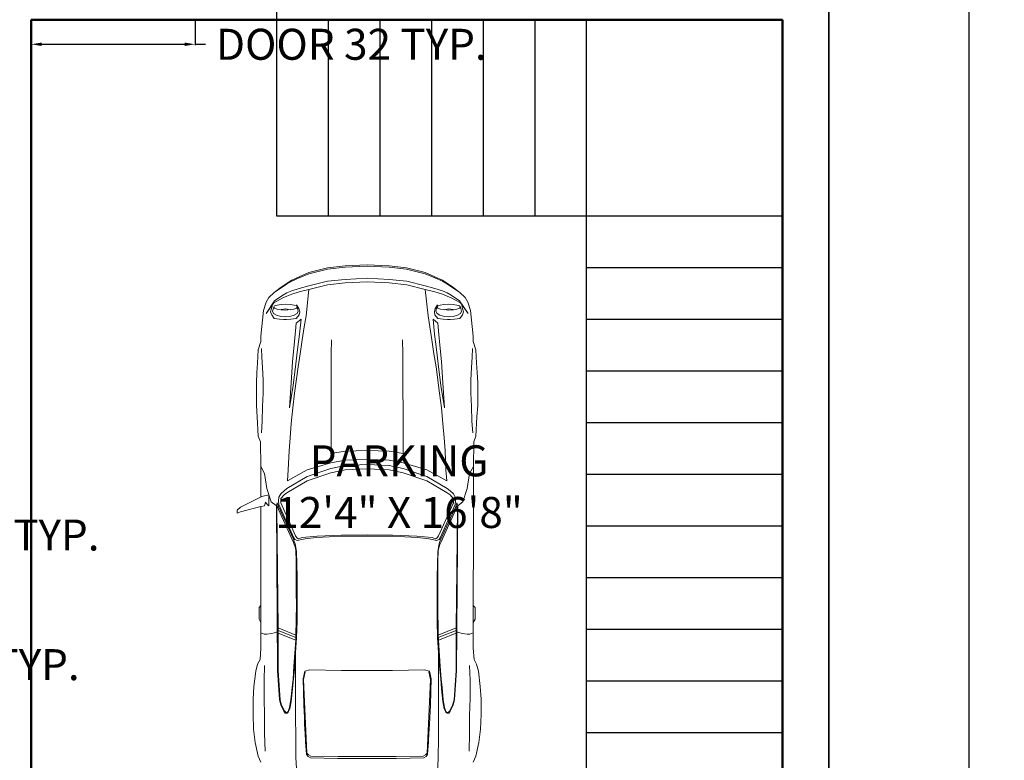
# Model space of a CAD drawing. Units: inches. Extents: x -20 to 10156, y 488 to 2970.
# Tile 3 of 6: x 221 to 412, y 581 to 724. Entities that reach past the tile are written whole.
import ezdxf

# ---------------------------------------------------------------- set-up
doc = ezdxf.new("R2010")
doc.units = ezdxf.units.IN
doc.header["$MEASUREMENT"] = 0
for name, color, linetype, lineweight in [('A-ANNO-DIMS', 2, 'Continuous', 18), ('A-AREA-IDEN', 7, 'Continuous', 25), ('A-FLOR-STRS', 7, 'Continuous', 25), ('A-FURN-VEHC', 8, 'Continuous', 13), ('A-WALL', 7, 'Continuous', 50), ('C-PROP', 7, 'Continuous', 35)]:
    doc.layers.add(name, color=color, linetype=linetype, lineweight=lineweight)
doc.styles.get("Standard").update_dxf_attribs({"font": 'arial.ttf'})
doc.dimstyles.get("Standard").update_dxf_attribs({"dimtxt": 6, "dimasz": 2, "dimexe": 0.18, "dimexo": 0.0625, "dimgap": 0.09, "dimtad": 0, "dimtih": 1, "dimtoh": 1, "dimdec": 0, "dimzin": 0, "dimdsep": 46, "dimlunit": 4, "dimtxsty": 'Standard', "dimcen": 0.09, "dimadec": 0, "dimazin": 0, "dimtfac": 1, "dimtdec": 0, "dimtofl": 0, "dimtmove": 0, "dimatfit": 3, "dimfxl": 1, "dimtolj": 1, "dimtzin": 0, "dimarcsym": 0})

# ---------------------------------------------------------------- blocks, each defined once
blk = doc.blocks.new('*D12')
at = {"layer": 'A-ANNO-DIMS', "color": 0, "lineweight": -2, "transparency": 16777216}
for p, q in [((223.3, 724.17), (223.3, 719.29)), ((255.01, 724.17), (255.01, 719.29)), ((225.3, 719.47), (253.01, 719.47)), ((255.01, 719.47), (257.01, 719.47))]:
    blk.add_line(p, q, dxfattribs=at)
at = {"layer": 'A-ANNO-DIMS', "color": 0, "transparency": 16777216}
for points in [[(225.3, 719.81), (225.3, 719.14), (223.3, 719.47)], [(253.01, 719.81), (253.01, 719.14), (255.01, 719.47)]]:
    blk.add_solid(points, dxfattribs=at)
at = {"layer": 'Defpoints', "color": 0, "transparency": 16777216}
for p in [(223.3, 724.23), (255.01, 724.23), (255.01, 719.47)]:
    blk.add_point(p, dxfattribs=at)
at = {"layer": 'A-ANNO-DIMS', "color": 0, "transparency": 16777216, "insert": (285.29, 719.47), "char_height": 6, "attachment_point": 5}
blk.add_mtext('\\A1;DOOR 32 TYP.', dxfattribs=at)
blk = doc.blocks.new('*D14')
at = {"layer": 'A-ANNO-DIMS', "color": 0, "lineweight": -2, "transparency": 16777216}
for p, q in [((206, 618.67), (211.91, 618.67)), ((211.73, 616.67), (211.73, 602.56)), ((211.73, 582.06), (211.73, 596.17)), ((206, 580.06), (211.91, 580.06))]:
    blk.add_line(p, q, dxfattribs=at)
at = {"layer": 'A-ANNO-DIMS', "color": 0, "transparency": 16777216}
for points in [[(211.4, 616.67), (212.07, 616.67), (211.73, 618.67)], [(211.4, 582.06), (212.07, 582.06), (211.73, 580.06)]]:
    blk.add_solid(points, dxfattribs=at)
at = {"layer": 'Defpoints', "color": 0, "transparency": 16777216}
for p in [(205.94, 618.67), (205.94, 580.06), (211.73, 580.06)]:
    blk.add_point(p, dxfattribs=at)
at = {"layer": 'A-ANNO-DIMS', "color": 0, "transparency": 16777216, "insert": (211.73, 599.36), "char_height": 6, "attachment_point": 5}
blk.add_mtext('\\A1;WC 39 TYP.', dxfattribs=at)
blk = doc.blocks.new('*D15')
at = {"layer": 'A-ANNO-DIMS', "color": 0, "lineweight": -2, "transparency": 16777216}
for p, q in [((181.78, 618.73), (181.78, 624.64)), ((183.78, 624.46), (203.94, 624.46)), ((205.94, 618.73), (205.94, 624.64)), ((205.94, 624.46), (207.94, 624.46))]:
    blk.add_line(p, q, dxfattribs=at)
at = {"layer": 'A-ANNO-DIMS', "color": 0, "transparency": 16777216}
for points in [[(183.78, 624.79), (183.78, 624.13), (181.78, 624.46)], [(203.94, 624.79), (203.94, 624.13), (205.94, 624.46)]]:
    blk.add_solid(points, dxfattribs=at)
at = {"layer": 'Defpoints', "color": 0, "transparency": 16777216}
for p in [(205.94, 624.46), (181.78, 618.67), (205.94, 618.67)]:
    blk.add_point(p, dxfattribs=at)
at = {"layer": 'A-ANNO-DIMS', "color": 0, "transparency": 16777216, "insert": (222.69, 624.46), "char_height": 6, "attachment_point": 5}
blk.add_mtext('\\A1;24 TYP.', dxfattribs=at)
blk = doc.blocks.new('*D29')
at = {"layer": 'A-ANNO-DIMS', "color": 0, "lineweight": -2, "transparency": 16777216}
for p, q in [((377.86, 1058.73), (405.13, 1058.73)), ((404.95, 1056.73), (404.95, 791.88)), ((404.95, 520.73), (404.95, 785.58)), ((377.86, 518.73), (405.13, 518.73))]:
    blk.add_line(p, q, dxfattribs=at)
at = {"layer": 'A-ANNO-DIMS', "color": 0, "transparency": 16777216}
for points in [[(404.62, 1056.73), (405.28, 1056.73), (404.95, 1058.73)], [(404.62, 520.73), (405.28, 520.73), (404.95, 518.73)]]:
    blk.add_solid(points, dxfattribs=at)
at = {"layer": 'Defpoints', "color": 0, "transparency": 16777216}
for p in [(377.8, 1058.73), (404.95, 1058.73), (377.8, 518.73)]:
    blk.add_point(p, dxfattribs=at)
at = {"layer": 'A-ANNO-DIMS', "color": 0, "transparency": 16777216, "insert": (404.95, 788.73), "char_height": 6, "attachment_point": 5}
blk.add_mtext('\\A1;540', dxfattribs=at)

msp = doc.modelspace()

# ---------------------------------------------------------------- linework, layer by layer
at = {"layer": 'A-FLOR-STRS'}
for p, q in [((270.8, 728.73), (270.8, 686.23)), ((280.8, 724.23), (280.8, 686.23)), ((290.8, 724.23), (290.8, 686.23)), ((300.8, 724.23), (300.8, 686.23)), ((310.8, 724.23), (310.8, 686.23)), ((320.8, 724.23), (320.8, 686.23)), ((330.8, 724.23), (330.8, 676.23)), ((270.8, 686.23), (368.8, 686.23)), ((330.8, 676.23), (368.8, 676.23)), ((330.8, 676.23), (330.8, 566.23)), ((330.8, 666.23), (368.8, 666.23)), ((330.8, 656.23), (368.8, 656.23)), ((330.8, 646.23), (368.8, 646.23)), ((330.8, 636.23), (368.8, 636.23)), ((330.8, 626.23), (368.8, 626.23)), ((330.8, 616.23), (368.8, 616.23)), ((330.8, 606.23), (368.8, 606.23)), ((330.8, 596.23), (368.8, 596.23)), ((330.8, 586.23), (368.8, 586.23))]:
    msp.add_line(p, q, dxfattribs=at)
at = {"layer": 'A-FURN-VEHC'}
for p, q in [((277.07, 675.28, -279.43), (275.2, 674.47, -279.43)), ((280.66, 676.17, -279.43), (277.07, 675.28, -279.43)), ((280.66, 675.92, -279.43), (277.07, 675.02, -279.43)), ((284.07, 676.56, -279.43), (280.66, 676.17, -279.43)), ((284.07, 676.3, -279.43), (280.66, 675.92, -279.43)), ((288.33, 676.77, -279.43), (284.07, 676.56, -279.43)), ((288.33, 676.52, -279.43), (284.07, 676.3, -279.43)), ((288.33, 676.77, -279.43), (288.33, 676.77, -279.43)), ((288.33, 676.77, -279.43), (292.59, 676.56, -279.43)), ((288.33, 676.52, -279.43), (292.59, 676.3, -279.43)), ((292.59, 676.56, -279.43), (296, 676.17, -279.43)), ((292.59, 676.3, -279.43), (296, 675.92, -279.43)), ((296, 676.17, -279.43), (299.59, 675.28, -279.43)), ((296, 675.92, -279.43), (299.59, 675.02, -279.43)), ((299.59, 675.28, -279.43), (301.46, 674.47, -279.43)), ((273.75, 673.83, -279.43), (271.71, 672.43, -279.43)), ((273.75, 673.58, -279.43), (272.72, 673.02, -279.43)), ((275.2, 674.47, -279.43), (273.75, 673.83, -279.43)), ((275.2, 674.22, -279.43), (273.75, 673.58, -279.43)), ((277.07, 675.02, -279.43), (275.2, 674.22, -279.43)), ((277.06, 672.68, -279.43), (280.65, 673.58, -279.43)), ((280.65, 673.58, -279.43), (284.06, 673.96, -279.43)), ((284.06, 673.27, -279.43), (280.65, 672.89, -279.43)), ((284.06, 673.96, -279.43), (288.33, 674.17, -279.43)), ((288.33, 673.48, -279.43), (284.06, 673.27, -279.43)), ((292.6, 673.96, -279.43), (288.33, 674.17, -279.43)), ((288.33, 673.48, -279.43), (292.6, 673.27, -279.43)), ((296.01, 673.58, -279.43), (292.6, 673.96, -279.43)), ((292.6, 673.27, -279.43), (296.01, 672.89, -279.43)), ((299.6, 672.68, -279.43), (296.01, 673.58, -279.43)), ((299.59, 675.02, -279.43), (301.46, 674.22, -279.43)), ((301.46, 674.47, -279.43), (302.92, 673.83, -279.43)), ((301.46, 674.22, -279.43), (302.92, 673.58, -279.43)), ((302.92, 673.83, -279.43), (304.95, 672.43, -279.43)), ((302.92, 673.58, -279.43), (303.94, 673.02, -279.43)), ((270.33, 671.4, -279.43), (269.31, 670.46, -279.43)), ((272.72, 673.02, -279.43), (270.33, 671.4, -279.43)), ((271.71, 672.43, -279.43), (270.33, 671.4, -279.43)), ((272.03, 670.89, -279.43), (272.79, 671.32, -279.43)), ((272.79, 671.32, -279.43), (273.73, 671.74, -279.43)), ((273.73, 671.74, -279.43), (275.19, 672.2, -279.43)), ((275.19, 671.53, -279.43), (273.73, 671.06, -279.43)), ((275.19, 672.2, -279.43), (277.06, 672.68, -279.43)), ((277.06, 671.99, -279.43), (275.19, 671.53, -279.43)), ((277.06, 671.99, -279.43), (276.53, 666.9, -279.43)), ((280.65, 672.89, -279.43), (277.06, 671.99, -279.43)), ((296.01, 672.89, -279.43), (299.6, 671.99, -279.43)), ((301.47, 672.2, -279.43), (299.6, 672.68, -279.43)), ((299.6, 671.99, -279.43), (301.47, 671.53, -279.43)), ((299.6, 671.99, -279.43), (300.14, 666.9, -279.43)), ((302.93, 671.74, -279.43), (301.47, 672.2, -279.43)), ((301.47, 671.53, -279.43), (302.93, 671.06, -279.43)), ((303.87, 671.32, -279.43), (302.93, 671.74, -279.43)), ((304.63, 670.89, -279.43), (303.87, 671.32, -279.43)), ((303.94, 673.02, -279.43), (306.33, 671.4, -279.43)), ((304.95, 672.43, -279.43), (306.33, 671.4, -279.43)), ((306.33, 671.4, -279.43), (307.35, 670.46, -279.43)), ((268.8, 669.53, -279.43), (268.29, 667.9, -279.43)), ((268.76, 667.37, -279.43), (270.4, 669.78, -279.43)), ((270.25, 669.43, -279.43), (268.76, 667.37, -279.43)), ((269.31, 670.46, -279.43), (268.8, 669.53, -279.43)), ((272.03, 670.38, -279.43), (270.25, 669.43, -279.43)), ((270.4, 669.78, -279.43), (272.03, 670.89, -279.43)), ((272.79, 670.71, -279.43), (272.03, 670.38, -279.43)), ((273.73, 671.06, -279.43), (272.79, 670.71, -279.43)), ((302.93, 671.06, -279.43), (303.87, 670.71, -279.43)), ((303.87, 670.71, -279.43), (304.63, 670.38, -279.43)), ((306.26, 669.78, -279.43), (304.63, 670.89, -279.43)), ((304.63, 670.38, -279.43), (306.41, 669.43, -279.43)), ((307.9, 667.37, -279.43), (306.26, 669.78, -279.43)), ((306.41, 669.43, -279.43), (307.9, 667.37, -279.43)), ((307.35, 670.46, -279.43), (307.86, 669.53, -279.43)), ((307.86, 669.53, -279.43), (308.38, 667.9, -279.43)), ((268.29, 667.9, -279.43), (267.77, 662.95, -279.43)), ((269.82, 668.33, -279.43), (269.66, 667.64, -279.43)), ((269.66, 667.64, -279.43), (269.87, 667.07, -279.43)), ((270, 669.01, -279.43), (269.82, 668.33, -279.43)), ((270.01, 667.78, -279.43), (270.25, 668.58, -279.43)), ((270.21, 667.35, -279.43), (270.01, 667.78, -279.43)), ((270.43, 668.8, -279.43), (270.25, 668.58, -279.43)), ((270.25, 668.58, -279.43), (270.43, 668.39, -279.43)), ((270.93, 668.98, -279.43), (270.43, 668.8, -279.43)), ((270.43, 668.39, -279.43), (270.93, 668.2, -279.43)), ((271.67, 669.11, -279.43), (270.93, 668.98, -279.43)), ((270.93, 668.2, -279.43), (271.6, 668.08, -279.43)), ((271.6, 668.08, -279.43), (272.56, 668.02, -279.43)), ((272.56, 669.14, -279.43), (271.67, 669.11, -279.43)), ((271.67, 668.11, -279.43), (272.56, 668.22, -279.43)), ((273.43, 669.11, -279.43), (272.56, 669.14, -279.43)), ((272.56, 668.22, -279.43), (273.42, 668.07, -279.43)), ((272.56, 668.02, -279.43), (273.43, 668.11, -279.43)), ((274.19, 668.98, -279.43), (273.43, 669.11, -279.43)), ((273.43, 668.11, -279.43), (274.13, 668.19, -279.43)), ((274.13, 668.19, -279.43), (274.64, 668.37, -279.43)), ((274.65, 668.8, -279.43), (274.19, 668.98, -279.43)), ((274.64, 668.37, -279.43), (274.8, 668.58, -279.43)), ((274.8, 668.58, -279.43), (274.65, 668.8, -279.43)), ((275.12, 668.33, -279.43), (274.69, 669.01, -279.43)), ((274.99, 667.78, -279.43), (274.77, 667.35, -279.43)), ((274.8, 668.58, -279.43), (274.94, 668.04, -279.43)), ((274.94, 668.04, -279.43), (274.99, 667.78, -279.43)), ((275.28, 667.64, -279.43), (275.12, 668.33, -279.43)), ((275.21, 667.07, -279.43), (275.28, 667.64, -279.43)), ((301.38, 667.64, -279.43), (301.54, 668.33, -279.43)), ((301.45, 667.07, -279.43), (301.38, 667.64, -279.43)), ((301.54, 668.33, -279.43), (301.97, 669.01, -279.43)), ((301.72, 668.04, -279.43), (301.67, 667.78, -279.43)), ((301.67, 667.78, -279.43), (301.89, 667.35, -279.43)), ((301.86, 668.58, -279.43), (301.72, 668.04, -279.43)), ((301.86, 668.58, -279.43), (302.01, 668.8, -279.43)), ((302.02, 668.37, -279.43), (301.86, 668.58, -279.43)), ((302.01, 668.8, -279.43), (302.48, 668.98, -279.43)), ((302.53, 668.19, -279.43), (302.02, 668.37, -279.43)), ((302.48, 668.98, -279.43), (303.23, 669.11, -279.43)), ((303.23, 668.11, -279.43), (302.53, 668.19, -279.43)), ((303.23, 669.11, -279.43), (304.1, 669.14, -279.43)), ((304.1, 668.02, -279.43), (303.23, 668.11, -279.43)), ((304.1, 668.22, -279.43), (303.24, 668.07, -279.43)), ((304.1, 669.14, -279.43), (304.99, 669.11, -279.43)), ((304.99, 668.11, -279.43), (304.1, 668.22, -279.43)), ((305.06, 668.08, -279.43), (304.1, 668.02, -279.43)), ((304.99, 669.11, -279.43), (305.73, 668.98, -279.43)), ((305.73, 668.2, -279.43), (305.06, 668.08, -279.43)), ((305.73, 668.98, -279.43), (306.24, 668.8, -279.43)), ((306.24, 668.39, -279.43), (305.73, 668.2, -279.43)), ((306.24, 668.8, -279.43), (306.41, 668.58, -279.43)), ((306.41, 668.58, -279.43), (306.24, 668.39, -279.43)), ((306.65, 667.78, -279.43), (306.41, 668.58, -279.43)), ((306.46, 667.35, -279.43), (306.65, 667.78, -279.43)), ((306.67, 669.01, -279.43), (306.84, 668.33, -279.43)), ((307, 667.64, -279.43), (306.79, 667.07, -279.43)), ((306.84, 668.33, -279.43), (307, 667.64, -279.43)), ((308.38, 667.9, -279.43), (308.89, 662.95, -279.43)), ((269.87, 667.07, -279.43), (270.33, 666.39, -279.43)), ((270.8, 667.01, -279.43), (270.21, 667.35, -279.43)), ((270.33, 666.39, -279.43), (271.36, 666.22, -279.43)), ((271.66, 666.78, -279.43), (270.8, 667.01, -279.43)), ((271.36, 666.22, -279.43), (272.21, 666.19, -279.43)), ((272.51, 666.7, -279.43), (271.66, 666.78, -279.43)), ((272.21, 666.19, -279.43), (272.72, 666.19, -279.43)), ((273.36, 666.78, -279.43), (272.51, 666.7, -279.43)), ((272.72, 666.19, -279.43), (273.58, 666.22, -279.43)), ((274.22, 667.01, -279.43), (273.36, 666.78, -279.43)), ((273.58, 666.22, -279.43), (274.61, 666.39, -279.43)), ((274.77, 667.35, -279.43), (274.22, 667.01, -279.43)), ((274.61, 666.39, -279.43), (275.21, 667.07, -279.43)), ((275.55, 666.24, -279.43), (274.62, 665.48, -279.43)), ((275.25, 663.32, -279.43), (275.55, 666.24, -279.43)), ((276.53, 666.9, -279.43), (276.18, 664.79, -279.43)), ((300.14, 666.9, -279.43), (300.48, 664.79, -279.43)), ((301.42, 663.32, -279.43), (301.11, 666.24, -279.43)), ((301.11, 666.24, -279.43), (302.04, 665.48, -279.43)), ((302.06, 666.39, -279.43), (301.45, 667.07, -279.43)), ((301.89, 667.35, -279.43), (302.44, 667.01, -279.43)), ((303.08, 666.22, -279.43), (302.06, 666.39, -279.43)), ((302.44, 667.01, -279.43), (303.3, 666.78, -279.43)), ((303.94, 666.19, -279.43), (303.08, 666.22, -279.43)), ((303.3, 666.78, -279.43), (304.15, 666.7, -279.43)), ((304.45, 666.19, -279.43), (303.94, 666.19, -279.43)), ((304.15, 666.7, -279.43), (305, 666.78, -279.43)), ((305.3, 666.22, -279.43), (304.45, 666.19, -279.43)), ((305, 666.78, -279.43), (305.86, 667.01, -279.43)), ((306.33, 666.39, -279.43), (305.3, 666.22, -279.43)), ((305.86, 667.01, -279.43), (306.46, 667.35, -279.43)), ((306.79, 667.07, -279.43), (306.33, 666.39, -279.43)), ((274.49, 663.96, -279.43), (274.22, 661.19, -279.43)), ((274.62, 665.48, -279.43), (274.49, 663.96, -279.43)), ((276.18, 664.79, -279.43), (275.78, 662.26, -279.43)), ((300.48, 664.79, -279.43), (300.88, 662.26, -279.43)), ((302.04, 665.48, -279.43), (302.17, 663.96, -279.43)), ((302.17, 663.96, -279.43), (302.44, 661.19, -279.43)), ((267.77, 661.92, -279.43), (267.27, 660.31, -279.43)), ((267.77, 662.95, -279.43), (267.77, 661.92, -279.43)), ((274.87, 660.4, -279.43), (275.25, 663.32, -279.43)), ((275.78, 662.26, -279.43), (275.37, 659.52, -279.43)), ((281.4, 659.52, -279.43), (281.44, 662.26, -279.43)), ((295.26, 659.52, -279.43), (295.22, 662.26, -279.43)), ((300.88, 662.26, -279.43), (301.29, 659.52, -279.43)), ((301.79, 660.4, -279.43), (301.42, 663.32, -279.43)), ((308.89, 662.95, -279.43), (308.89, 661.92, -279.43)), ((308.89, 661.92, -279.43), (309.39, 660.31, -279.43)), ((267.27, 660.31, -279.43), (267.12, 657.75, -279.43)), ((267.89, 660.56, -279.43), (267.97, 658.86, -279.43)), ((274.22, 661.19, -279.43), (273.92, 658.03, -279.43)), ((274.54, 657.57, -279.43), (274.87, 660.4, -279.43)), ((302.13, 657.57, -279.43), (301.79, 660.4, -279.43)), ((302.44, 661.19, -279.43), (302.74, 658.03, -279.43)), ((308.77, 660.56, -279.43), (308.69, 658.86, -279.43)), ((309.39, 660.31, -279.43), (309.54, 657.75, -279.43)), ((267.97, 658.86, -279.43), (268.09, 656.9, -279.43)), ((273.92, 658.03, -279.43), (273.7, 654.86, -279.43)), ((275.37, 659.52, -279.43), (274.97, 657.05, -279.43)), ((281.35, 641.81, -279.43), (281.4, 659.52, -279.43)), ((295.32, 641.81, -279.43), (295.26, 659.52, -279.43)), ((301.29, 659.52, -279.43), (301.7, 657.05, -279.43)), ((302.74, 658.03, -279.43), (302.96, 654.86, -279.43)), ((308.69, 658.86, -279.43), (308.57, 656.9, -279.43)), ((267.12, 657.75, -279.43), (266.98, 655.95, -279.43)), ((268.09, 656.9, -279.43), (268.2, 654.43, -279.43)), ((274.05, 653.4, -279.43), (274.54, 657.57, -279.43)), ((274.97, 657.05, -279.43), (274.28, 651.95, -279.43)), ((301.7, 657.05, -279.43), (302.38, 651.95, -279.43)), ((302.61, 653.4, -279.43), (302.13, 657.57, -279.43)), ((308.57, 656.9, -279.43), (308.46, 654.43, -279.43)), ((309.54, 657.75, -279.43), (309.68, 655.95, -279.43)), ((266.98, 655.95, -279.43), (266.9, 653.92, -279.43)), ((268.2, 654.43, -279.43), (268.23, 651.95, -279.43)), ((273.7, 654.86, -279.43), (273.31, 649.05, -279.43)), ((302.96, 654.86, -279.43), (303.35, 649.05, -279.43)), ((308.46, 654.43, -279.43), (308.44, 651.95, -279.43)), ((309.68, 655.95, -279.43), (309.76, 653.92, -279.43)), ((266.9, 653.92, -279.43), (266.9, 651.95, -279.43)), ((273.31, 649.05, -279.43), (274.05, 653.4, -279.43)), ((303.35, 649.05, -279.43), (302.61, 653.4, -279.43)), ((309.76, 653.92, -279.43), (309.76, 651.95, -279.43)), ((266.9, 651.95, -279.43), (266.9, 649.56, -279.43)), ((268.23, 651.95, -279.43), (268.11, 649.34, -279.43)), ((274.28, 651.95, -279.43), (273.94, 649.05, -279.43)), ((302.38, 651.95, -279.43), (302.72, 649.05, -279.43)), ((308.44, 651.95, -279.43), (308.55, 649.34, -279.43)), ((309.76, 651.95, -279.43), (309.76, 649.56, -279.43)), ((266.9, 649.56, -279.43), (267.04, 647.34, -279.43)), ((268.11, 649.34, -279.43), (268.03, 646.49, -279.43)), ((273.94, 649.05, -279.43), (273.66, 646.06, -279.43)), ((302.72, 649.05, -279.43), (303, 646.06, -279.43)), ((308.55, 649.34, -279.43), (308.63, 646.49, -279.43)), ((309.76, 649.56, -279.43), (309.62, 647.34, -279.43)), ((267.04, 647.34, -279.43), (267.27, 643.59, -279.43)), ((309.62, 647.34, -279.43), (309.39, 643.59, -279.43)), ((268.03, 646.49, -279.43), (267.87, 644.24, -279.43)), ((273.66, 646.06, -279.43), (273.41, 643.25, -279.43)), ((303, 646.06, -279.43), (303.25, 643.25, -279.43)), ((308.63, 646.49, -279.43), (308.8, 644.24, -279.43)), ((267.27, 643.59, -279.43), (267.67, 642.47, -279.43)), ((273.41, 643.25, -279.43), (273.23, 640.77, -279.43)), ((303.25, 643.25, -279.43), (303.43, 640.77, -279.43)), ((309.39, 643.59, -279.43), (308.99, 642.47, -279.43)), ((267.67, 642.47, -279.43), (267.74, 637.7, -279.43)), ((281.33, 640.25, -279.43), (281.35, 641.81, -279.43)), ((288.33, 640.84, -279.43), (284.07, 640.67, -279.43)), ((288.33, 640.84, -279.43), (292.59, 640.67, -279.43)), ((295.33, 640.25, -279.43), (295.32, 641.81, -279.43)), ((308.99, 642.47, -279.43), (308.92, 637.7, -279.43)), ((273.23, 640.77, -279.43), (273.07, 637.08, -279.43)), ((284.07, 640.67, -279.43), (281.33, 640.25, -279.43)), ((281.33, 638.41, -279.43), (284.07, 638.92, -279.43)), ((284.07, 638.92, -279.43), (288.33, 639.1, -279.43)), ((292.59, 638.92, -279.43), (288.33, 639.1, -279.43)), ((292.59, 640.67, -279.43), (295.33, 640.25, -279.43)), ((295.33, 638.41, -279.43), (292.59, 638.92, -279.43)), ((303.43, 640.77, -279.43), (303.59, 637.08, -279.43)), ((267.74, 637.7, -279.43), (267.73, 631.8, -279.43)), ((268.46, 636.34, -279.43), (267.74, 637.7, -279.43)), ((273.07, 637.08, -279.43), (272.9, 634.93, -279.43)), ((272.9, 634.93, -279.43), (276.73, 637.05, -279.43)), ((276.73, 637.05, -279.43), (281.33, 638.41, -279.43)), ((281.33, 637.34, -279.43), (276.73, 635.8, -279.43)), ((284.07, 637.93, -279.43), (281.33, 637.34, -279.43)), ((284.07, 637.07, -279.43), (281.33, 636.48, -279.43)), ((288.33, 638.11, -279.43), (284.07, 637.93, -279.43)), ((288.33, 637.25, -279.43), (284.07, 637.07, -279.43)), ((288.33, 638.11, -279.43), (292.59, 637.93, -279.43)), ((288.33, 637.25, -279.43), (292.59, 637.07, -279.43)), ((292.59, 637.93, -279.43), (295.33, 637.34, -279.43)), ((292.59, 637.07, -279.43), (295.33, 636.48, -279.43)), ((299.94, 637.05, -279.43), (295.33, 638.41, -279.43)), ((295.33, 637.34, -279.43), (299.94, 635.8, -279.43)), ((303.77, 634.93, -279.43), (299.94, 637.05, -279.43)), ((303.59, 637.08, -279.43), (303.77, 634.93, -279.43)), ((308.2, 636.34, -279.43), (308.92, 637.7, -279.43)), ((308.92, 637.7, -279.43), (308.94, 631.8, -279.43)), ((268.91, 633.44, -279.43), (268.46, 636.34, -279.43)), ((276.73, 635.8, -279.43), (272.81, 633.44, -279.43)), ((281.33, 636.48, -279.43), (276.73, 634.94, -279.43)), ((295.33, 636.48, -279.43), (299.94, 634.94, -279.43)), ((299.94, 635.8, -279.43), (303.85, 633.44, -279.43)), ((307.75, 633.44, -279.43), (308.2, 636.34, -279.43)), ((269.78, 630.88, -279.43), (268.91, 633.44, -279.43)), ((272.81, 633.44, -279.43), (272.25, 633.03, -279.43)), ((276.73, 634.94, -279.43), (272.81, 632.61, -279.43)), ((299.94, 634.94, -279.43), (303.85, 632.61, -279.43)), ((303.85, 633.44, -279.43), (304.41, 633.03, -279.43)), ((306.89, 630.88, -279.43), (307.75, 633.44, -279.43)), ((267.95, 631.9, -279.43), (263.85, 629.85, -279.43)), ((269.31, 632.24, -279.43), (267.95, 631.9, -279.43)), ((269.31, 630.11, -279.43), (269.31, 632.24, -279.43)), ((271.27, 631.77, -279.43), (271.21, 631.1, -279.43)), ((271.61, 632.41, -279.43), (271.27, 631.77, -279.43)), ((271.66, 631.55, -279.43), (271.6, 630.68, -279.43)), ((272.25, 633.03, -279.43), (271.61, 632.41, -279.43)), ((272.25, 632.24, -279.43), (271.66, 631.55, -279.43)), ((272.81, 632.61, -279.43), (272.25, 632.24, -279.43)), ((303.85, 632.61, -279.43), (304.41, 632.24, -279.43)), ((304.41, 633.03, -279.43), (305.05, 632.41, -279.43)), ((304.41, 632.24, -279.43), (305, 631.55, -279.43)), ((305, 631.55, -279.43), (305.06, 630.68, -279.43)), ((305.05, 632.41, -279.43), (305.4, 631.77, -279.43)), ((305.4, 631.77, -279.43), (305.46, 631.1, -279.43)), ((308.92, 629.96, -279.43), (308.94, 631.8, -279.43)), ((263.85, 629.85, -279.43), (263.18, 629.26, -279.43)), ((263.85, 628.92, -279.43), (267.75, 629.96, -279.43)), ((267.74, 629.96, -279.43), (267.78, 605.55, -279.43)), ((267.75, 629.96, -279.43), (268.46, 630.13, -279.43)), ((268.46, 630.13, -279.43), (268.63, 630.8, -279.43)), ((268.63, 630.8, -279.43), (269.04, 630.3, -279.43)), ((269.04, 630.3, -279.43), (269.31, 630.11, -279.43)), ((270.7, 630.19, -279.43), (269.78, 630.88, -279.43)), ((270.76, 630.19, -279.43), (270.94, 630.67, -279.43)), ((271.01, 598.2, -279.43), (270.76, 630.19, -279.43)), ((270.85, 629.82, -279.43), (270.94, 630.08, -279.43)), ((270.97, 617.72, -279.43), (270.85, 629.82, -279.43)), ((270.94, 630.67, -279.43), (271.16, 630.01, -279.43)), ((270.94, 630.08, -279.43), (271.16, 629.4, -279.43)), ((271.16, 630.01, -279.43), (274.06, 623.65, -279.43)), ((271.16, 629.4, -279.43), (274.06, 623.04, -279.43)), ((271.21, 631.1, -279.43), (271.23, 630.37, -279.43)), ((271.23, 630.37, -279.43), (274.15, 623.94, -279.43)), ((271.6, 630.68, -279.43), (274.5, 624.29, -279.43)), ((305.06, 630.68, -279.43), (302.16, 624.29, -279.43)), ((305.43, 630.37, -279.43), (302.51, 623.94, -279.43)), ((305.5, 630.01, -279.43), (302.6, 623.65, -279.43)), ((305.5, 629.4, -279.43), (302.6, 623.04, -279.43)), ((305.46, 631.1, -279.43), (305.43, 630.37, -279.43)), ((305.72, 630.67, -279.43), (305.5, 630.01, -279.43)), ((305.72, 630.08, -279.43), (305.5, 629.4, -279.43)), ((305.65, 598.2, -279.43), (305.9, 630.19, -279.43)), ((305.69, 617.72, -279.43), (305.82, 629.82, -279.43)), ((305.9, 630.19, -279.43), (305.72, 630.67, -279.43)), ((305.82, 629.82, -279.43), (305.72, 630.08, -279.43)), ((305.97, 630.19, -279.43), (306.89, 630.88, -279.43)), ((308.92, 629.96, -279.43), (308.88, 605.55, -279.43)), ((263.18, 629.26, -279.43), (263.18, 628.67, -279.43)), ((263.18, 628.67, -279.43), (263.85, 628.92, -279.43)), ((274.06, 623.65, -279.43), (274.22, 623.22, -279.43)), ((274.15, 623.94, -279.43), (274.35, 623.56, -279.43)), ((274.5, 624.29, -279.43), (274.73, 623.91, -279.43)), ((274.73, 623.91, -279.43), (275.05, 623.75, -279.43)), ((275.05, 623.75, -279.43), (275.75, 623.95, -279.43)), ((275.65, 623.56, -279.43), (276.73, 623.77, -279.43)), ((275.75, 623.95, -279.43), (278.67, 624.25, -279.43)), ((276.73, 623.77, -279.43), (278.61, 623.99, -279.43)), ((278.61, 623.99, -279.43), (283.4, 624.23, -279.43)), ((278.67, 624.25, -279.43), (283.4, 624.44, -279.43)), ((283.4, 624.44, -279.43), (288.33, 624.48, -279.43)), ((283.4, 624.23, -279.43), (288.33, 624.21, -279.43)), ((293.27, 624.44, -279.43), (288.33, 624.48, -279.43)), ((293.27, 624.23, -279.43), (288.33, 624.21, -279.43)), ((297.99, 624.25, -279.43), (293.27, 624.44, -279.43)), ((298.05, 623.99, -279.43), (293.27, 624.23, -279.43)), ((300.92, 623.95, -279.43), (297.99, 624.25, -279.43)), ((299.94, 623.77, -279.43), (298.05, 623.99, -279.43)), ((301.01, 623.56, -279.43), (299.94, 623.77, -279.43)), ((301.61, 623.75, -279.43), (300.92, 623.95, -279.43)), ((301.93, 623.91, -279.43), (301.61, 623.75, -279.43)), ((302.16, 624.29, -279.43), (301.93, 623.91, -279.43)), ((302.51, 623.94, -279.43), (302.31, 623.56, -279.43)), ((302.6, 623.65, -279.43), (302.44, 623.22, -279.43)), ((274.06, 623.04, -279.43), (274.22, 622.61, -279.43)), ((274.22, 623.22, -279.43), (274.39, 622.75, -279.43)), ((274.22, 622.61, -279.43), (274.39, 622.15, -279.43)), ((274.35, 623.56, -279.43), (274.85, 623.39, -279.43)), ((274.39, 622.75, -279.43), (274.65, 621.27, -279.43)), ((274.39, 622.15, -279.43), (274.55, 621.52, -279.43)), ((274.85, 623.39, -279.43), (275.65, 623.56, -279.43)), ((301.81, 623.39, -279.43), (301.01, 623.56, -279.43)), ((302.31, 623.56, -279.43), (301.81, 623.39, -279.43)), ((302.28, 622.75, -279.43), (302.01, 621.27, -279.43)), ((302.28, 622.15, -279.43), (302.11, 621.52, -279.43)), ((302.44, 623.22, -279.43), (302.28, 622.75, -279.43)), ((302.44, 622.61, -279.43), (302.28, 622.15, -279.43)), ((302.6, 623.04, -279.43), (302.44, 622.61, -279.43)), ((274.55, 621.52, -279.43), (274.62, 619.32, -279.43)), ((274.65, 621.27, -279.43), (274.77, 616.37, -279.43)), ((302.01, 621.27, -279.43), (301.89, 616.37, -279.43)), ((302.11, 621.52, -279.43), (302.04, 619.32, -279.43)), ((274.62, 619.32, -279.43), (274.62, 616.39, -279.43)), ((302.04, 619.32, -279.43), (302.04, 616.39, -279.43)), ((271.1, 606.48, -279.43), (270.97, 617.72, -279.43)), ((274.62, 616.39, -279.43), (274.63, 613.28, -279.43)), ((274.77, 616.37, -279.43), (274.77, 611.01, -279.43)), ((301.89, 616.37, -279.43), (301.89, 611.01, -279.43)), ((302.04, 616.39, -279.43), (302.03, 613.28, -279.43)), ((305.56, 606.48, -279.43), (305.69, 617.72, -279.43)), ((274.63, 613.28, -279.43), (274.65, 611, -279.43)), ((302.03, 613.28, -279.43), (302.01, 611, -279.43)), ((267.76, 610.83, -279.43), (267.42, 610.4, -279.43)), ((267.42, 610.4, -279.43), (267.42, 608.19, -279.43)), ((267.76, 611.01, -279.43), (267.76, 610.83, -279.43)), ((274.65, 611, -279.43), (274.56, 605.09, -279.43)), ((274.77, 611.01, -279.43), (274.77, 607.79, -279.43)), ((301.89, 611.01, -279.43), (301.89, 607.79, -279.43)), ((302.01, 611, -279.43), (302.1, 605.09, -279.43)), ((308.9, 611.01, -279.43), (308.9, 610.83, -279.43)), ((308.9, 610.83, -279.43), (309.24, 610.4, -279.43)), ((309.24, 610.4, -279.43), (309.24, 608.19, -279.43)), ((267.42, 608.19, -279.43), (267.76, 607.5, -279.43)), ((267.76, 607.5, -279.43), (267.76, 606.57, -279.43)), ((271.1, 606.48, -279.43), (274.56, 605.09, -279.43)), ((271.1, 605.63, -279.43), (271.1, 606.48, -279.43)), ((274.77, 607.79, -279.43), (274.68, 604.53, -279.43)), ((301.89, 607.79, -279.43), (301.98, 604.53, -279.43)), ((305.56, 606.48, -279.43), (302.1, 605.09, -279.43)), ((305.56, 605.63, -279.43), (305.56, 606.48, -279.43)), ((309.24, 608.19, -279.43), (308.9, 607.5, -279.43)), ((308.9, 607.5, -279.43), (308.9, 606.57, -279.43)), ((267.78, 605.55, -279.43), (267.77, 602.53, -279.43)), ((268.43, 605.29, -279.43), (267.78, 605.55, -279.43)), ((268.95, 605.29, -279.43), (268.43, 605.29, -279.43)), ((269.9, 605.37, -279.43), (268.95, 605.29, -279.43)), ((270.76, 605.63, -279.43), (269.9, 605.37, -279.43)), ((271.1, 605.63, -279.43), (270.76, 605.63, -279.43)), ((271.09, 598.2, -279.43), (271.1, 605.63, -279.43)), ((271.1, 605.98, -279.43), (274.54, 604.59, -279.43)), ((271.1, 605.48, -279.43), (274.51, 604.1, -279.43)), ((274.56, 605.09, -279.43), (274.51, 604.09, -279.43)), ((302.1, 605.09, -279.43), (302.15, 604.09, -279.43)), ((305.56, 605.98, -279.43), (302.13, 604.59, -279.43)), ((305.56, 605.48, -279.43), (302.15, 604.1, -279.43)), ((305.57, 598.2, -279.43), (305.56, 605.63, -279.43)), ((305.56, 605.63, -279.43), (305.9, 605.63, -279.43)), ((305.9, 605.63, -279.43), (306.76, 605.37, -279.43)), ((306.76, 605.37, -279.43), (307.71, 605.29, -279.43)), ((307.71, 605.29, -279.43), (308.24, 605.29, -279.43)), ((308.24, 605.29, -279.43), (308.88, 605.55, -279.43)), ((308.88, 605.55, -279.43), (308.89, 602.53, -279.43)), ((274.51, 604.09, -279.43), (274.18, 599.06, -279.43)), ((274.68, 604.53, -279.43), (274.49, 601.71, -279.43)), ((301.98, 604.53, -279.43), (302.17, 601.71, -279.43)), ((302.15, 604.09, -279.43), (302.49, 599.06, -279.43)), ((267.77, 602.53, -279.43), (267.61, 600.34, -279.43)), ((274.49, 601.71, -279.43), (274.32, 599.06, -279.43)), ((274.49, 601.71, -279.43), (274.47, 589.51, -279.43)), ((302.17, 601.71, -279.43), (302.35, 599.06, -279.43)), ((302.17, 601.71, -279.43), (302.2, 589.51, -279.43)), ((308.89, 602.53, -279.43), (309.05, 600.34, -279.43)), ((267.1, 599.48, -279.43), (266.76, 598.12, -279.43)), ((267.61, 600.34, -279.43), (267.1, 599.48, -279.43)), ((268.48, 599.17, -279.43), (268.38, 596.35, -279.43)), ((274.18, 599.06, -279.43), (274, 596.58, -279.43)), ((274.32, 599.06, -279.43), (274.07, 596.6, -279.43)), ((302.35, 599.06, -279.43), (302.6, 596.6, -279.43)), ((302.49, 599.06, -279.43), (302.66, 596.58, -279.43)), ((308.19, 599.17, -279.43), (308.28, 596.35, -279.43)), ((309.05, 600.34, -279.43), (309.56, 599.48, -279.43)), ((309.56, 599.48, -279.43), (309.9, 598.12, -279.43)), ((266.76, 598.12, -279.43), (266.41, 595.14, -279.43)), ((271.38, 592.58, -279.43), (271.01, 598.2, -279.43)), ((271.49, 592.57, -279.43), (271.09, 598.2, -279.43)), ((276.26, 598.12, -279.43), (275.95, 596.6, -279.43)), ((276.04, 596.48, -279.43), (276.35, 598, -279.43)), ((277.24, 598.38, -279.43), (276.26, 598.12, -279.43)), ((283.38, 598.21, -279.43), (277.24, 598.38, -279.43)), ((288.34, 598.2, -279.43), (283.38, 598.21, -279.43)), ((288.32, 598.2, -279.43), (293.28, 598.21, -279.43)), ((293.28, 598.21, -279.43), (299.43, 598.38, -279.43)), ((299.43, 598.38, -279.43), (300.4, 598.12, -279.43)), ((300.62, 596.48, -279.43), (300.31, 598, -279.43)), ((300.4, 598.12, -279.43), (300.72, 596.6, -279.43)), ((305.18, 592.57, -279.43), (305.57, 598.2, -279.43)), ((305.28, 592.58, -279.43), (305.65, 598.2, -279.43)), ((309.9, 598.12, -279.43), (310.25, 595.14, -279.43)), ((266.41, 595.14, -279.43), (266.25, 592.66, -279.43)), ((268.38, 596.35, -279.43), (268.38, 592.86, -279.43)), ((274, 596.58, -279.43), (273.81, 594.91, -279.43)), ((274.07, 596.6, -279.43), (273.9, 594.68, -279.43)), ((275.95, 596.6, -279.43), (275.99, 594.15, -279.43)), ((276.69, 582.24, -279.43), (276.04, 596.48, -279.43)), ((299.97, 582.24, -279.43), (300.62, 596.48, -279.43)), ((300.72, 596.6, -279.43), (300.67, 594.15, -279.43)), ((302.6, 596.6, -279.43), (302.76, 594.68, -279.43)), ((302.66, 596.58, -279.43), (302.85, 594.91, -279.43)), ((308.28, 596.35, -279.43), (308.28, 592.86, -279.43)), ((310.25, 595.14, -279.43), (310.41, 592.66, -279.43)), ((273.81, 594.91, -279.43), (273.58, 592.56, -279.43)), ((273.9, 594.68, -279.43), (273.62, 592.24, -279.43)), ((275.99, 594.15, -279.43), (276.07, 591.5, -279.43)), ((300.67, 594.15, -279.43), (300.59, 591.5, -279.43)), ((302.76, 594.68, -279.43), (303.04, 592.24, -279.43)), ((302.85, 594.91, -279.43), (303.08, 592.56, -279.43)), ((266.25, 592.66, -279.43), (266.25, 589.68, -279.43)), ((268.38, 592.86, -279.43), (268.48, 589.53, -279.43)), ((271.65, 591.49, -279.43), (271.38, 592.58, -279.43)), ((271.78, 591.53, -279.43), (271.49, 592.57, -279.43)), ((272.22, 590.32, -279.43), (271.65, 591.49, -279.43)), ((272.31, 590.44, -279.43), (271.78, 591.53, -279.43)), ((273.58, 592.56, -279.43), (273.34, 591.03, -279.43)), ((273.62, 592.24, -279.43), (273.37, 590.78, -279.43)), ((276.07, 591.5, -279.43), (276.19, 589.15, -279.43)), ((300.59, 591.5, -279.43), (300.47, 589.15, -279.43)), ((303.04, 592.24, -279.43), (303.29, 590.78, -279.43)), ((303.08, 592.56, -279.43), (303.32, 591.03, -279.43)), ((304.35, 590.44, -279.43), (304.88, 591.53, -279.43)), ((304.44, 590.32, -279.43), (305.01, 591.49, -279.43)), ((304.88, 591.53, -279.43), (305.18, 592.57, -279.43)), ((305.01, 591.49, -279.43), (305.28, 592.58, -279.43)), ((308.28, 592.86, -279.43), (308.19, 589.53, -279.43)), ((310.41, 592.66, -279.43), (310.41, 589.68, -279.43)), ((266.25, 589.68, -279.43), (266.33, 586.86, -279.43)), ((268.48, 589.53, -279.43), (268.48, 586.08, -279.43)), ((272.49, 589.97, -279.43), (272.22, 590.32, -279.43)), ((272.57, 590.13, -279.43), (272.31, 590.44, -279.43)), ((272.84, 589.94, -279.43), (272.49, 589.97, -279.43)), ((272.85, 590.12, -279.43), (272.57, 590.13, -279.43)), ((273.07, 590.17, -279.43), (272.84, 589.94, -279.43)), ((273.07, 590.3, -279.43), (272.85, 590.12, -279.43)), ((273.34, 591.03, -279.43), (273.07, 590.3, -279.43)), ((273.37, 590.78, -279.43), (273.07, 590.17, -279.43)), ((274.47, 589.51, -279.43), (274.51, 585.15, -279.43)), ((302.2, 589.51, -279.43), (302.15, 585.15, -279.43)), ((303.29, 590.78, -279.43), (303.59, 590.17, -279.43)), ((303.32, 591.03, -279.43), (303.59, 590.3, -279.43)), ((303.59, 590.3, -279.43), (303.81, 590.12, -279.43)), ((303.59, 590.17, -279.43), (303.83, 589.94, -279.43)), ((303.81, 590.12, -279.43), (304.09, 590.13, -279.43)), ((303.83, 589.94, -279.43), (304.17, 589.97, -279.43)), ((304.09, 590.13, -279.43), (304.35, 590.44, -279.43)), ((304.17, 589.97, -279.43), (304.44, 590.32, -279.43)), ((308.19, 589.53, -279.43), (308.19, 586.08, -279.43)), ((310.41, 589.68, -279.43), (310.33, 586.86, -279.43)), ((276.19, 589.15, -279.43), (276.24, 587.78, -279.43)), ((276.24, 587.78, -279.43), (276.34, 586.03, -279.43)), ((300.43, 587.78, -279.43), (300.32, 586.03, -279.43)), ((300.47, 589.15, -279.43), (300.43, 587.78, -279.43)), ((266.33, 586.86, -279.43), (266.67, 584.3, -279.43)), ((268.48, 586.08, -279.43), (268.57, 582.63, -279.43)), ((276.34, 586.03, -279.43), (276.43, 584.47, -279.43)), ((300.32, 586.03, -279.43), (300.23, 584.47, -279.43)), ((308.19, 586.08, -279.43), (308.09, 582.63, -279.43)), ((310.33, 586.86, -279.43), (310, 584.3, -279.43)), ((266.67, 584.3, -279.43), (267.26, 581.66, -279.43)), ((274.51, 585.15, -279.43), (274.56, 581.4, -279.43)), ((276.43, 584.47, -279.43), (276.6, 581.95, -279.43)), ((300.23, 584.47, -279.43), (300.07, 581.95, -279.43)), ((302.15, 585.15, -279.43), (302.1, 581.4, -279.43)), ((310, 584.3, -279.43), (309.4, 581.66, -279.43)), ((276.6, 581.95, -279.43), (276.9, 581.59, -279.43)), ((276.98, 581.88, -279.43), (276.69, 582.24, -279.43)), ((277.45, 581.61, -279.43), (276.98, 581.88, -279.43)), ((299.22, 581.61, -279.43), (299.68, 581.88, -279.43)), ((299.68, 581.88, -279.43), (299.97, 582.24, -279.43)), ((300.07, 581.95, -279.43), (299.76, 581.59, -279.43)), ((267.26, 581.66, -279.43), (267.75, 580.46, -279.43)), ((274.56, 581.4, -279.43), (274.7, 578.21, -279.43)), ((276.9, 581.59, -279.43), (277.35, 581.31, -279.43)), ((277.35, 581.31, -279.43), (282.63, 581.22, -279.43)), ((282.71, 581.56, -279.43), (277.45, 581.61, -279.43)), ((282.63, 581.22, -279.43), (288.33, 581.22, -279.43)), ((288.34, 581.56, -279.43), (282.71, 581.56, -279.43)), ((288.32, 581.56, -279.43), (293.95, 581.56, -279.43)), ((294.04, 581.22, -279.43), (288.33, 581.22, -279.43)), ((293.95, 581.56, -279.43), (299.22, 581.61, -279.43)), ((299.31, 581.31, -279.43), (294.04, 581.22, -279.43)), ((299.76, 581.59, -279.43), (299.31, 581.31, -279.43)), ((302.1, 581.4, -279.43), (301.96, 578.21, -279.43)), ((309.4, 581.66, -279.43), (308.91, 580.46, -279.43))]:
    msp.add_line(p, q, dxfattribs=at)
at = {"layer": 'A-WALL'}
for p, q in [((223.3, 527.73), (223.3, 724.23)), ((223.3, 724.23), (368.8, 724.23)), ((368.8, 724.23), (368.8, 527.73))]:
    msp.add_line(p, q, dxfattribs=at)
at = {"layer": 'C-PROP'}
msp.add_line((377.8, 1058.73), (377.8, 518.73), dxfattribs=at)

# ---------------------------------------------------------------- texts
at = {"layer": 'A-AREA-IDEN', "insert": (247.87, 641.82), "char_height": 6, "attachment_point": 1}
msp.add_mtext_dynamic_manual_height_columns('\\pxqc;PARKING\\P12\'4" X 16\'8"', width=93.3452, gutter_width=30, heights=[0], dxfattribs=at)

# ---------------------------------------------------------------- dimensions: what is measured, and where the dimension line sits
at = {"layer": 'A-ANNO-DIMS'}
dim = msp.add_linear_dim(base=(404.95, 1058.73), p1=(377.8, 518.73), p2=(377.8, 1058.73), angle=90, dimstyle='Standard', override={"dimdec": 0, "dimlfac": 1, "dimrnd": 0, "dimzin": 0, "dimdsep": 46, "dimlunit": 2}, dxfattribs=at)
dim.commit()
dim.dimension.update_dxf_attribs({"geometry": '*D29', "text_midpoint": (404.95, 788.73)})
for base, p1, p2, text, picture, middle in [((255.01, 719.47), (223.3, 724.23), (255.01, 724.23), 'DOOR <> TYP.', '*D12', (285.29, 719.47)), ((205.94, 624.46), (181.78, 618.67), (205.94, 618.67), '<> TYP.', '*D15', (222.69, 624.46))]:
    dim = msp.add_linear_dim(base=base, p1=p1, p2=p2, text=text, dimstyle='Standard', override={"dimdec": 0, "dimlfac": 1, "dimrnd": 0, "dimzin": 0, "dimdsep": 46, "dimlunit": 2}, dxfattribs=at)
    dim.commit()
    dim.dimension.update_dxf_attribs({"geometry": picture, "text_midpoint": middle})
dim = msp.add_linear_dim(base=(211.73, 580.06), p1=(205.94, 618.67), p2=(205.94, 580.06), angle=270, text='WC <> TYP.', dimstyle='Standard', override={"dimdec": 0, "dimlfac": 1, "dimrnd": 0, "dimzin": 0, "dimdsep": 46, "dimlunit": 2}, dxfattribs=at)
dim.commit()
dim.dimension.update_dxf_attribs({"geometry": '*D14', "text_midpoint": (211.73, 599.36)})

doc.saveas('drawing.dxf')
